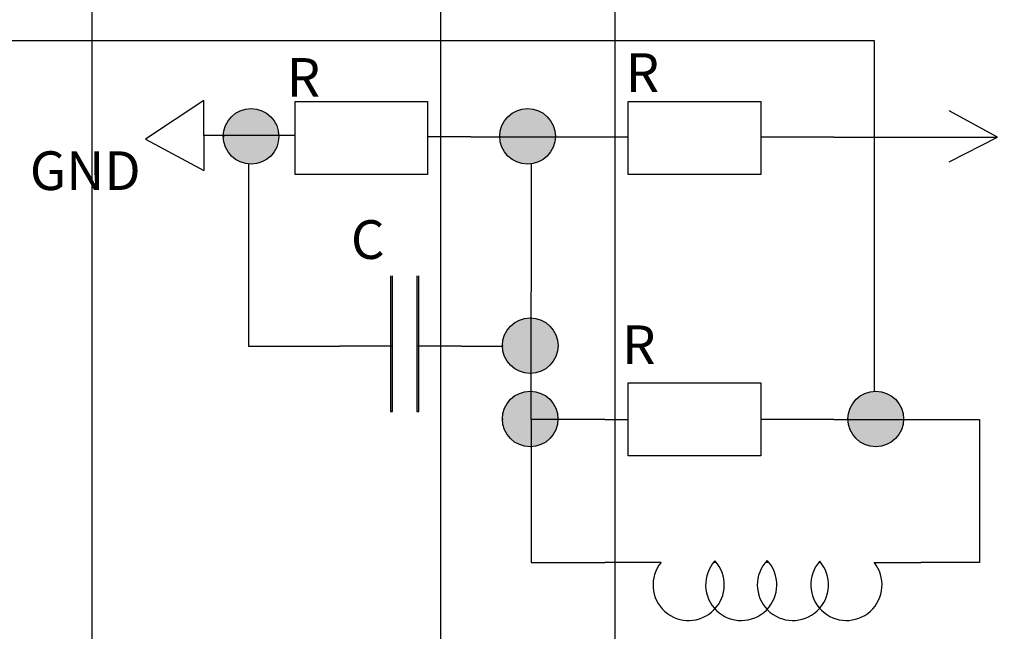
# Model space of a CAD drawing. Units: inches. Extents: x 35362 to 73946, y 43607 to 67532.
# Tile 133 of 134: x 64925 to 70544, y 46290 to 49781. Entities that reach past the tile are written whole.
import ezdxf

# ---------------------------------------------------------------- set-up
doc = ezdxf.new("R2010")
doc.units = ezdxf.units.IN
doc.header["$MEASUREMENT"] = 0
for name, color, linetype, lineweight in [('A-ANNO-DIMS', 2, 'Continuous', 18), ('E-ANNO-TEXT', 5, 'Continuous', 18), ('E-SYMB', 1, 'Continuous', 25), ('E-SYMB-PATT', 1, 'Continuous', 13), ('E-WIRE', 3, 'Continuous', 25)]:
    doc.layers.add(name, color=color, linetype=linetype, lineweight=lineweight)
doc.styles.get("Standard").update_dxf_attribs({"font": 'arial.ttf'})
doc.dimstyles.get("Standard").update_dxf_attribs({"dimtxt": 0.18, "dimasz": 0.18, "dimexe": 0.18, "dimexo": 0.0625, "dimgap": 0.09, "dimtad": 0, "dimtih": 1, "dimtoh": 1, "dimdec": 4, "dimzin": 0, "dimdsep": 46, "dimtxsty": 'Standard', "dimcen": 0.09, "dimadec": 0, "dimazin": 0, "dimtfac": 1, "dimtdec": 4, "dimtofl": 0, "dimtmove": 0, "dimatfit": 3, "dimfxl": 1, "dimtolj": 1, "dimtzin": 0, "dimarcsym": 0})

# ---------------------------------------------------------------- blocks, each defined once
blk = doc.blocks.new('PWR-5V')
for p, q in [((149.83075954589, 1350.920325582869), (-0.0001436721213395, 1075.898385659784)), ((149.83075954589, 833.0941938853575), (149.83075954589, 1350.920325582869)), ((289.9554714129044, 1075.898385659784), (149.83075954589, 1350.920325582869)), ((149.83075954589, 416.3126341884199), (149.83075954589, 833.0941938853575)), ((149.83075954589, 416.3126341884199), (149.83075954589, 0.0003315384019515))]:
    blk.add_line(p, q)
blk = doc.blocks.new('*D5')
at = {"layer": 'A-ANNO-DIMS', "color": 0, "lineweight": -2, "transparency": 16777216}
for p, q in [((37121.949085, 46919.318283), (37121.949085, 43606.678996)), ((69871.496302, 45449.831951), (69871.496302, 43606.678996)), ((37122.129085, 43606.858996), (53496.2943647142, 43606.858996)), ((69871.316302, 43606.858996), (53497.15102228581, 43606.858996))]:
    blk.add_line(p, q, dxfattribs=at)
at = {"layer": 'A-ANNO-DIMS', "color": 0, "transparency": 16777216}
for points in [[(37122.129085, 43606.888996), (37122.129085, 43606.828996), (37121.949085, 43606.858996)], [(69871.316302, 43606.888996), (69871.316302, 43606.828996), (69871.496302, 43606.858996)]]:
    blk.add_solid(points, dxfattribs=at)
at = {"layer": 'Defpoints', "color": 0, "transparency": 16777216}
for p in [(37121.949085, 46919.380783), (69871.496302, 45449.894451), (69871.496302, 43606.858996)]:
    blk.add_point(p, dxfattribs=at)
at = {"layer": 'A-ANNO-DIMS', "color": 0, "transparency": 16777216, "insert": (53496.7226935, 43606.858996), "char_height": 0.18, "attachment_point": 5}
blk.add_mtext('\\A1;32750', dxfattribs=at)
blk = doc.blocks.new('*D6')
at = {"layer": 'A-ANNO-DIMS', "color": 0, "lineweight": -2, "transparency": 16777216}
for p, q in [((72185.645666, 53702.123839), (72185.645666, 43606.678996)), ((69871.496302, 45449.831951), (69871.496302, 43606.678996)), ((69871.67630199999, 43606.858996), (71028.21104539152, 43606.858996)), ((72185.465666, 43606.858996), (71028.93092260844, 43606.858996))]:
    blk.add_line(p, q, dxfattribs=at)
at = {"layer": 'A-ANNO-DIMS', "color": 0, "transparency": 16777216}
for points in [[(69871.67630199999, 43606.888996), (69871.67630199999, 43606.828996), (69871.496302, 43606.858996)], [(72185.465666, 43606.888996), (72185.465666, 43606.828996), (72185.645666, 43606.858996)]]:
    blk.add_solid(points, dxfattribs=at)
at = {"layer": 'Defpoints', "color": 0, "transparency": 16777216}
for p in [(72185.645666, 53702.186339), (69871.496302, 45449.894451), (72185.645666, 43606.858996)]:
    blk.add_point(p, dxfattribs=at)
at = {"layer": 'A-ANNO-DIMS', "color": 0, "transparency": 16777216, "insert": (71028.57098399999, 43606.858996), "char_height": 0.18, "attachment_point": 5}
blk.add_mtext('\\A1;2314', dxfattribs=at)
blk = doc.blocks.new('*D7')
at = {"layer": 'A-ANNO-DIMS', "color": 0, "lineweight": -2, "transparency": 16777216}
for p, q in [((72185.70816600003, 53702.18633900003), (73945.82566600003, 53702.18633900003)), ((73945.64566600005, 53702.00633900003), (73945.64566600005, 49576.22229813781)), ((73945.64566600005, 45450.07445100001), (73945.64566600005, 49575.85849186223)), ((69871.55880200003, 45449.89445100001), (73945.82566600003, 45449.89445100001))]:
    blk.add_line(p, q, dxfattribs=at)
at = {"layer": 'A-ANNO-DIMS', "color": 0, "transparency": 16777216}
for points in [[(73945.61566600006, 53702.00633900003), (73945.67566600005, 53702.00633900003), (73945.64566600005, 53702.18633900003)], [(73945.61566600006, 45450.07445100001), (73945.67566600005, 45450.07445100001), (73945.64566600005, 45449.89445100001)]]:
    blk.add_solid(points, dxfattribs=at)
at = {"layer": 'Defpoints', "color": 0, "transparency": 16777216}
for p in [(72185.64566600003, 53702.18633900003), (73945.64566600005, 53702.18633900003), (69871.49630200001, 45449.89445100001)]:
    blk.add_point(p, dxfattribs=at)
at = {"layer": 'A-ANNO-DIMS', "color": 0, "transparency": 16777216, "insert": (73945.64566600005, 49576.04039499998), "char_height": 0.18, "attachment_point": 5}
blk.add_mtext('\\A1;8252', dxfattribs=at)
blk = doc.blocks.new('*D65')
at = {"layer": 'A-ANNO-DIMS', "color": 0, "lineweight": -2, "transparency": 16777216}
for p, q in [((65336.01600799999, 61293.223552), (65336.01600799999, 43606.678996)), ((67326.639741, 61293.223552), (67326.639741, 43606.678996)), ((65336.19600799999, 43606.858996), (66330.87277900206, 43606.858996)), ((67326.45974100001, 43606.858996), (66331.78296999796, 43606.858996))]:
    blk.add_line(p, q, dxfattribs=at)
at = {"layer": 'A-ANNO-DIMS', "color": 0, "transparency": 16777216}
for points in [[(65336.19600799999, 43606.888996), (65336.19600799999, 43606.828996), (65336.01600799999, 43606.858996)], [(67326.45974100001, 43606.888996), (67326.45974100001, 43606.828996), (67326.639741, 43606.858996)]]:
    blk.add_solid(points, dxfattribs=at)
at = {"layer": 'Defpoints', "color": 0, "transparency": 16777216}
for p in [(65336.01600799999, 61293.286052), (67326.639741, 61293.286052), (67326.639741, 43606.858996)]:
    blk.add_point(p, dxfattribs=at)
at = {"layer": 'A-ANNO-DIMS', "color": 0, "transparency": 16777216, "insert": (66331.32787450001, 43606.858996), "char_height": 0.18, "attachment_point": 5}
blk.add_mtext('\\A1;1990.6', dxfattribs=at)
blk = doc.blocks.new('*D68')
at = {"layer": 'A-ANNO-DIMS', "color": 0, "lineweight": -2, "transparency": 16777216}
for p, q in [((68320.870762, 54372.885224), (68320.870762, 43606.678996)), ((61240.907336, 53351.466162), (61240.907336, 43606.678996)), ((61241.08733599999, 43606.858996), (64780.42646373397, 43606.858996)), ((68320.69076200001, 43606.858996), (64781.35163426603, 43606.858996))]:
    blk.add_line(p, q, dxfattribs=at)
at = {"layer": 'A-ANNO-DIMS', "color": 0, "transparency": 16777216}
for points in [[(61241.08733599999, 43606.888996), (61241.08733599999, 43606.828996), (61240.907336, 43606.858996)], [(68320.69076200001, 43606.888996), (68320.69076200001, 43606.828996), (68320.870762, 43606.858996)]]:
    blk.add_solid(points, dxfattribs=at)
at = {"layer": 'Defpoints', "color": 0, "transparency": 16777216}
for p in [(68320.870762, 54372.947724), (61240.907336, 53351.52866199999), (68320.870762, 43606.858996)]:
    blk.add_point(p, dxfattribs=at)
at = {"layer": 'A-ANNO-DIMS', "color": 0, "transparency": 16777216, "insert": (64780.889049, 43606.858996), "char_height": 0.18, "attachment_point": 5}
blk.add_mtext('\\A1;7080.0', dxfattribs=at)

msp = doc.modelspace()

# ---------------------------------------------------------------- hatches: boundary and pattern name
at = {"layer": 'E-SYMB-PATT'}
h = msp.add_hatch(color=256, dxfattribs=at)
h.dxf.hatch_style = 1
h.paths.add_polyline_path([(66404.12963541549, 49112.54682942698, 0.4183931940818975), (66245.53985003696, 49273.41262076414, 0.4183931940818975), (66086.95006465843, 49112.54682942698)])
h.paths.add_polyline_path([(66404.12963541549, 49112.54682942698), (66086.95006465843, 49112.54682942698, 0.4100462469397049), (66245.53985003696, 48956.20084798897, 0.4100462469397049)])
h = msp.add_hatch(color=256, dxfattribs=at)
h.dxf.hatch_style = 1
h.paths.add_polyline_path([(67982.01794069535, 49112.54682942698, 0.4183931940818975), (67823.42815531684, 49273.41262076414, 0.4183931940818975), (67664.83836993828, 49112.54682942698)])
h.paths.add_polyline_path([(67982.01794069535, 49112.54682942698), (67664.83836993828, 49112.54682942698, 0.4100462469397049), (67823.42815531684, 48956.20084798897, 0.4100462469397049)])
h = msp.add_hatch(color=256, dxfattribs=at)
h.dxf.hatch_style = 1
h.paths.add_polyline_path([(67041.26428785537, 47544.13389292191), (67052.41899758835, 47544.13389292191), (67052.41899758835, 48318.26861425332), (67041.26428785537, 48318.26861425332)])
h = msp.add_hatch(color=256, dxfattribs=at)
h.dxf.hatch_style = 1
h.paths.add_polyline_path([(67192.22576528155, 47544.13389292191), (67203.38047501454, 47544.13389292191), (67203.38047501454, 48318.26861425332), (67192.22576528155, 48318.26861425332)])
h = msp.add_hatch(color=256, dxfattribs=at)
h.dxf.hatch_style = 1
h.paths.add_polyline_path([(67997.23375700117, 47918.08884068267, 0.4183931940818975), (67838.64397162265, 48078.95463201982, 0.4183931940818975), (67680.0541862441, 47918.08884068267)])
h.paths.add_polyline_path([(67997.23375700117, 47918.08884068267), (67680.0541862441, 47918.08884068267, 0.4100462469397049), (67838.64397162265, 47761.74285924466, 0.4100462469397049)])
h = msp.add_hatch(color=256, dxfattribs=at)
h.dxf.hatch_style = 1
h.paths.add_polyline_path([(67996.94821318585, 47499.73482830046, 0.4183931940818975), (67838.35842780732, 47660.60061963762, 0.4183931940818975), (67679.76864242878, 47499.73482830046)])
h.paths.add_polyline_path([(67996.94821318585, 47499.73482830046), (67679.76864242878, 47499.73482830046, 0.4100462469397049), (67838.35842780732, 47343.38884686247, 0.4100462469397049)])
h = msp.add_hatch(color=256, dxfattribs=at)
h.dxf.hatch_style = 1
h.paths.add_polyline_path([(69969.39519919358, 47499.73482830045, 0.4183931940818975), (69810.80541381503, 47660.60061963761, 0.4183931940818975), (69652.2156284365, 47499.73482830045)])
h.paths.add_polyline_path([(69969.39519919358, 47499.73482830045), (69652.2156284365, 47499.73482830045, 0.4100462469397049), (69810.80541381503, 47343.38884686245, 0.4100462469397049)])

# ---------------------------------------------------------------- linework, layer by layer
at = {"layer": 'E-SYMB'}
for p, q in [((65975.45730067026, 49320.0791314712), (65642.52431800886, 49098.36844373563)), ((65975.45730067026, 49120.07913147119), (65975.45730067026, 49320.0791314712)), ((66404.05807935355, 49120.07913147119), (65975.45730067026, 49120.07913147119)), ((65975.45730067026, 49120.07913147119), (65975.45730067026, 48920.0791314712)), ((66404.12883500017, 49117.12212745924), (66403.44261173914, 49117.12212745924)), ((66496.37891909842, 49120.07913147119), (66404.05807935355, 49120.07913147119)), ((67982.01714028005, 49117.12212745924), (67981.330917019, 49117.12212745924)), ((65642.52431800886, 49098.36844373563), (65975.45730067026, 48920.0791314712)), ((66091.42121014332, 49112.54682942698), (66086.95006465843, 49112.54682942698)), ((67500.29642789123, 49112.54682942698), (67252.99721277317, 49112.54682942698)), ((67669.30951542319, 49112.54682942698), (67664.83836993828, 49112.54682942698)), ((68127.52752583481, 49112.54682942698), (68397.64321966901, 49112.54682942698)), ((67041.26428785537, 48318.26861425332), (67041.26428785537, 47544.13389292191)), ((67052.41899758835, 47544.13389292191), (67052.41899758835, 48318.26861425332)), ((67192.22576528155, 48318.26861425332), (67192.22576528155, 47544.13389292191)), ((67203.38047501454, 47544.13389292191), (67203.38047501454, 48318.26861425332)), ((67052.41899758835, 47918.08884068266), (66750.86385828078, 47918.08884068267)), ((67446.45940677969, 47918.08884068267), (67192.22576528155, 47918.08884068266)), ((67684.525331729, 47918.08884068267), (67680.0541862441, 47918.08884068267)), ((67997.23295658585, 47922.66413871493), (67996.54673332481, 47922.66413871493)), ((67041.26428785537, 47544.13389292191), (67052.41899758835, 47544.13389292191)), ((67192.22576528155, 47544.13389292191), (67203.38047501454, 47544.13389292191)), ((67684.23978791368, 47499.73482830046), (67679.76864242878, 47499.73482830046)), ((67996.94741277053, 47504.31012633272), (67996.26118950949, 47504.31012633272)), ((68264.72489034168, 47499.73482830046), (68397.64321966901, 47499.14132536252)), ((69570.57381599379, 47499.73482830045), (69154.26151334376, 47499.73482830045)), ((69656.6867739214, 47499.73482830045), (69652.2156284365, 47499.73482830045)), ((69969.39439877825, 47504.31012633271), (69968.70817551721, 47504.31012633271)), ((68387.4226745263, 46683.62309270856), (68264.72489034168, 46683.62309270856)), ((68585.03971847038, 46683.62309270856), (68387.4226745263, 46683.62309270856)), ((68900.48382237619, 46683.62309270856), (68885.22041349059, 46683.62309270856)), ((69200.66451739638, 46683.62309270856), (69180.31324149497, 46683.62309270856)), ((69495.75734540077, 46683.62309270856), (69485.58170745008, 46683.62309270856)), ((69801.02581135588, 46683.62309270856), (70067.22750252108, 46683.62309270856))]:
    msp.add_line(p, q, dxfattribs=at)
for points in [[(67252.99721277317, 49314.66935503323), (67252.99721277317, 48897.73823615334), (66496.37891909842, 48897.73823615334), (66496.37891909842, 49314.66935503323)], [(69154.26151334376, 49314.66935503323), (69154.26151334376, 48897.73823615334), (68397.64321966901, 48897.73823615334), (68397.64321966901, 49314.66935503323)], [(69154.26151334376, 47708.2164545283), (69154.26151334376, 47291.28533564841), (68397.64321966901, 47291.28533564841), (68397.64321966901, 47708.2164545283)]]:
    msp.add_lwpolyline(points, close=True, dxfattribs=at)
for centre in [(66245.53985003696, 49114.80673437655), (67823.42815531684, 49114.80673437655), (67838.64397162265, 47920.34874563224), (67838.35842780732, 47501.99473325004), (69810.80541381503, 47501.99473325003)]:
    msp.add_circle(centre, 158.6058863875805, dxfattribs=at)
for centre, start, end in [((68742.76177042328, 46555.29343386573), 140.8666685730917, 42.42623157986281), ((69042.94246544348, 46555.29343386573), 137.5737684201371, 43.47826481578429), ((69338.03529344784, 46555.29343386573), 136.5217351842157, 41.35264262444016), ((69643.30375940297, 46555.29343386573), 138.6473573755598, 39.13333142690828)]:
    msp.add_arc(centre, 203.3340773479672, start, end, dxfattribs=at)
at = {"layer": 'E-WIRE'}
for p, q in [((69802.97030670266, 49659.17196353646), (64391.6881470991, 49659.17196353645)), ((69802.97030670266, 47660.40697486451), (69802.97030670266, 49659.17196353646)), ((67500.29642789123, 49112.54682942698), (68127.52752583481, 49112.54682942698)), ((66230.41345625285, 48956.9238049387), (66230.41345625285, 47918.08884068269)), ((67844.70994498099, 47499.73482830046), (67845.70511604888, 48957.77309397637)), ((66230.41345625285, 47918.08884068269), (66750.86385828078, 47918.08884068267)), ((67446.45940677969, 47918.08884068267), (67680.0541862441, 47918.08884068267)), ((68264.72489034168, 47499.73482830046), (67844.70994498099, 47499.73482830046)), ((67844.70994498099, 47499.73482830046), (67844.70994498099, 46683.62309270856)), ((69570.57381599379, 47499.73482830045), (69987.35537569072, 47499.73482830045)), ((69987.35537569072, 47499.73482830045), (70402.10124121375, 47499.73482830045)), ((70402.10124121375, 47499.73482830045), (70402.10124121375, 46683.62309270856)), ((67844.70994498099, 46683.62309270856), (68264.72489034168, 46683.62309270856)), ((70402.10124121375, 46683.62309270856), (70067.22750252108, 46683.62309270856))]:
    msp.add_line(p, q, dxfattribs=at)

# ---------------------------------------------------------------- block references
at = {"layer": 'E-SYMB', "rotation": 270.0000000000005}
msp.add_blockref('PWR-5V', (69154.26118180538, 49259.93511724339), dxfattribs=at)

# ---------------------------------------------------------------- texts
at = {"layer": 'E-ANNO-TEXT'}
for s, p in [('R', (68383.63435381863, 49368.21384313978)), ('R', (66448.85625166487, 49340.59836547636)), ('GND', (64982.83518931685, 48808.52662090376)), ('C', (66815.0820254838, 48415.47979169633)), ('R', (68362.9045457574, 47814.84304443391))]:
    msp.add_text(s, height=220.8659825270206, dxfattribs=at).set_placement(p)

# ---------------------------------------------------------------- dimensions: what is measured, and where the dimension line sits
at = {"layer": 'A-ANNO-DIMS'}
for base, p1, p2, override, picture, middle in [((67326.639741, 43606.858996), (65336.01600799999, 61293.286052), (67326.639741, 61293.286052), {"dimdec": 1, "dimlfac": 1, "dimrnd": 0, "dimzin": 0, "dimdsep": 46, "dimlunit": 2}, '*D65', (66331.32787450001, 43606.858996)), ((68320.870762, 43606.858996), (61240.907336, 53351.52866199999), (68320.870762, 54372.947724), {"dimdec": 1, "dimlfac": 1, "dimrnd": 0, "dimzin": 0, "dimdsep": 46, "dimlunit": 2}, '*D68', (64780.889049, 43606.858996)), ((72185.645666, 43606.858996), (69871.496302, 45449.894451), (72185.645666, 53702.186339), {"dimdec": 0, "dimlfac": 1, "dimrnd": 0, "dimzin": 0, "dimdsep": 46, "dimlunit": 2}, '*D6', (71028.57098399999, 43606.858996)), ((69871.496302, 43606.858996), (37121.949085, 46919.380783), (69871.496302, 45449.894451), {"dimdec": 0, "dimlfac": 1, "dimrnd": 0, "dimzin": 0, "dimdsep": 46, "dimlunit": 2}, '*D5', (53496.7226935, 43606.858996))]:
    dim = msp.add_linear_dim(base=base, p1=p1, p2=p2, dimstyle='Standard', override=override, dxfattribs=at)
    dim.commit()
    dim.dimension.update_dxf_attribs({"geometry": picture, "text_midpoint": middle})
dim = msp.add_linear_dim(base=(73945.64566600005, 53702.18633900003), p1=(69871.496302, 45449.894451), p2=(72185.645666, 53702.186339), angle=90, dimstyle='Standard', override={"dimdec": 0, "dimlfac": 1, "dimrnd": 0, "dimzin": 0, "dimdsep": 46, "dimlunit": 2}, dxfattribs=at)
dim.commit()
dim.dimension.update_dxf_attribs({"geometry": '*D7', "text_midpoint": (73945.64566600005, 49576.04039499998)})

doc.saveas('drawing.dxf')
